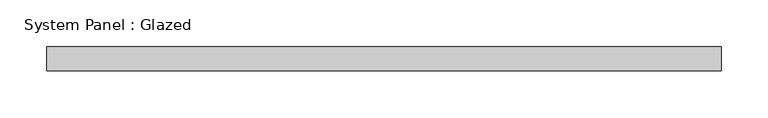
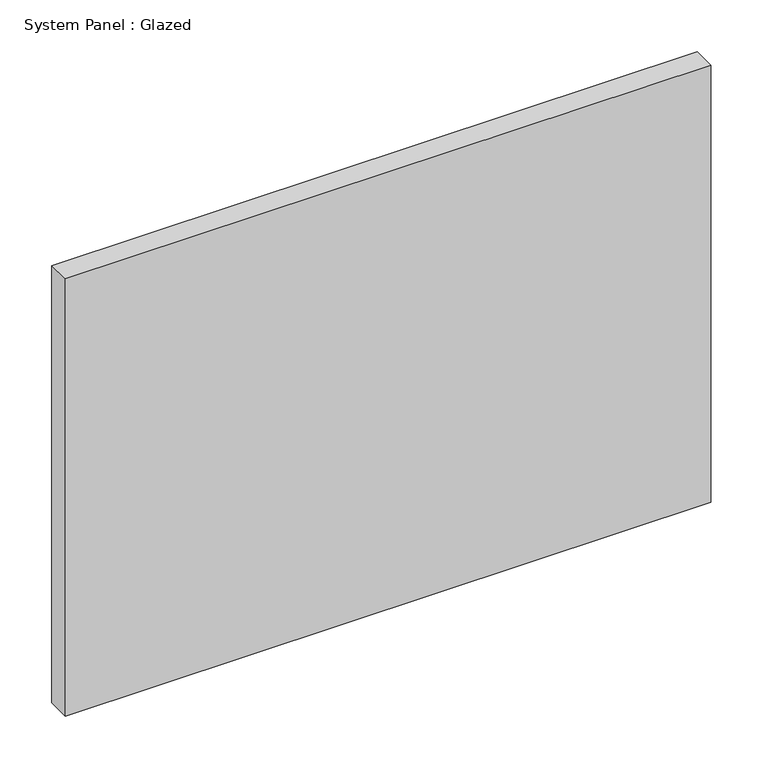
"""IFC4 building model written with IfcOpenShell, lengths in millimetres: plate geometry, System Panel : Glazed."""

from ifc_helpers import new_model, si_unit, origin, origin_with_axes, place, context, project, spatial, polyline, outline, extrude, source, transform, mapped, element, save


def system_panel_glazed_ce1d5741(model_context):
    return source(origin(), model_context, "Body", "SweptSolid", [
        extrude(outline(polyline([(358.775, 19.05), (-358.775, 19.05), (-358.775, 44.45), (358.775, 44.45), (358.775, 19.05)])), origin_with_axes(), (0.0, 0.0, 1.0), 513.9497047),
    ])


if __name__ == "__main__":
    model = new_model("IFC4")
    model_context = context("Model", 3, world=origin())
    ifc_project = project(units=[si_unit("LENGTHUNIT", "METRE", prefix="MILLI")], contexts=[model_context])
    site = spatial("IfcSite", under=ifc_project)
    building = spatial("IfcBuilding", under=site)
    placement = place(None, origin())
    system_panel_glazed_shape = system_panel_glazed_ce1d5741(model_context)
    element("IfcPlate", 1, ObjectType="System Panel : Glazed", at=placement, inside=building, context=model_context, shape_type="MappedRepresentation", body=[
        mapped(system_panel_glazed_shape, transform((0.0, 0.0, 0.0), x_axis=(1.0, 0.0, 0.0), y_axis=(0.0, 1.0, 0.0), z_axis=(0.0, 0.0, 1.0))),
    ])
    save(model, "model.ifc")

# Revit data of these elements
# Type "System Panel : Glazed"
#   Construction Type Id = "GSP4R"
#   Analytic Construction = "1/8 in Pilkington single glazing"
#   Visual Light Transmittance = 0.9
#   Solar Heat Gain Coefficient = 0.86
#   Heat Transfer Coefficient (U) = 1.18115 BTU/(h·ft²·°F)
#   Define Thermal Properties by = 1
# Element 1 (IfcPlate, "System Panel : Glazed")
#   Materials on its faces: "Glass"
# Materials
#   "Glass": class "Glass", colour RGB 0 128 192, transparency 0.75, Description = "Soda Lime Glass", Cost = 0
